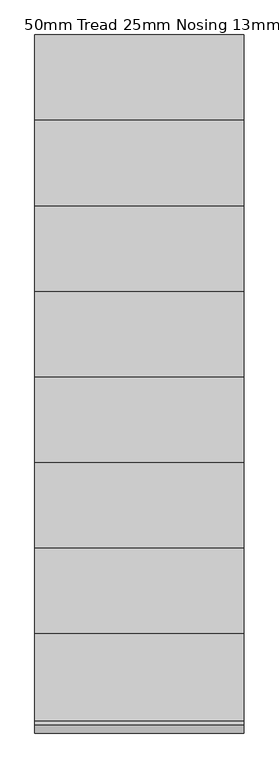
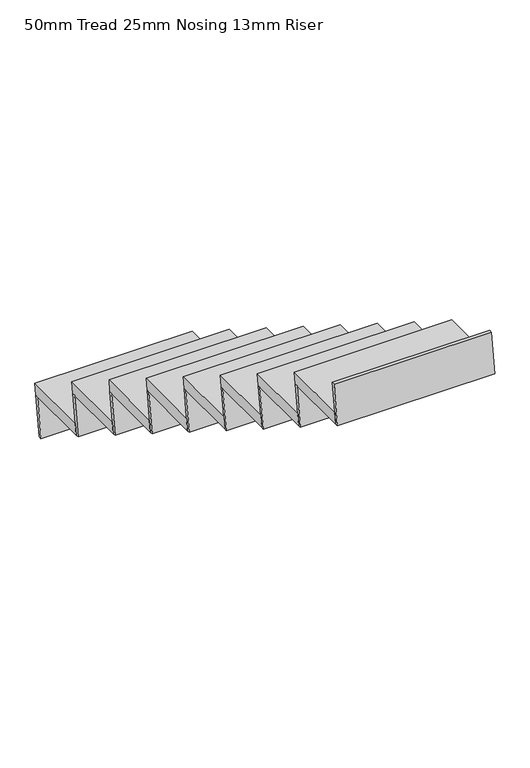
"""IFC4 building model written with IfcOpenShell, lengths in millimetres: stair flight geometry, 50mm Tread 25mm Nosing 13mm Riser."""

from ifc_helpers import new_model, si_unit, frame, origin, place, context, project, spatial, polyline, outline, extrude, source, transform, mapped, element, save


def stair_flight_50mm_tread_25mm_nosing_13mm_riser_fd2cf019(model_context):
    return source(origin(), model_context, "Body", "SweptSolid", [
        extrude(outline(polyline([(7051.2805518, 1913.0434783), (7351.2805518, 1913.0434783), (7344.0930518, 1863.0434783), (7044.0930518, 1863.0434783), (7051.2805518, 1913.0434783)])), frame((602.1868738, 0.0, 0.0), z_axis=(1.0, 0.0, 0.0), x_axis=(0.0, 1.0, 0.0)), (0.0, 0.0, 1.0), 673.3917263),
        extrude(outline(polyline([(7344.0930518, 1863.0434783), (7319.0930518, 1689.1304348), (7306.4645618, 1689.1304348), (7331.4645618, 1863.0434783), (7344.0930518, 1863.0434783)])), frame((602.1868738, 0.0, 0.0), z_axis=(1.0, 0.0, 0.0), x_axis=(0.0, 1.0, 0.0)), (0.0, 0.0, 1.0), 673.3917263),
        extrude(outline(polyline([(7069.0930518, 2036.9565217), (7044.0930518, 1863.0434783), (7031.4645618, 1863.0434783), (7056.4645618, 2036.9565217), (7069.0930518, 2036.9565217)])), frame((602.1868738, 0.0, 0.0), z_axis=(1.0, 0.0, 0.0), x_axis=(0.0, 1.0, 0.0)), (0.0, 0.0, 1.0), 673.3917263),
        extrude(outline(polyline([(6776.2805518, 2086.9565217), (7076.2805518, 2086.9565217), (7069.0930518, 2036.9565217), (6769.0930518, 2036.9565217), (6776.2805518, 2086.9565217)])), frame((602.1868738, 0.0, 0.0), z_axis=(1.0, 0.0, 0.0), x_axis=(0.0, 1.0, 0.0)), (0.0, 0.0, 1.0), 673.3917263),
        extrude(outline(polyline([(6794.0930518, 2210.8695652), (6769.0930518, 2036.9565217), (6756.4645618, 2036.9565217), (6781.4645618, 2210.8695652), (6794.0930518, 2210.8695652)])), frame((602.1868738, 0.0, 0.0), z_axis=(1.0, 0.0, 0.0), x_axis=(0.0, 1.0, 0.0)), (0.0, 0.0, 1.0), 673.3917263),
        extrude(outline(polyline([(6501.2805518, 2260.8695652), (6801.2805518, 2260.8695652), (6794.0930518, 2210.8695652), (6494.0930518, 2210.8695652), (6501.2805518, 2260.8695652)])), frame((602.1868738, 0.0, 0.0), z_axis=(1.0, 0.0, 0.0), x_axis=(0.0, 1.0, 0.0)), (0.0, 0.0, 1.0), 673.3917263),
        extrude(outline(polyline([(6519.0930518, 2384.7826087), (6494.0930518, 2210.8695652), (6481.4645618, 2210.8695652), (6506.4645618, 2384.7826087), (6519.0930518, 2384.7826087)])), frame((602.1868738, 0.0, 0.0), z_axis=(1.0, 0.0, 0.0), x_axis=(0.0, 1.0, 0.0)), (0.0, 0.0, 1.0), 673.3917263),
        extrude(outline(polyline([(6226.2805518, 2434.7826087), (6526.2805518, 2434.7826087), (6519.0930518, 2384.7826087), (6219.0930518, 2384.7826087), (6226.2805518, 2434.7826087)])), frame((602.1868738, 0.0, 0.0), z_axis=(1.0, 0.0, 0.0), x_axis=(0.0, 1.0, 0.0)), (0.0, 0.0, 1.0), 673.3917263),
        extrude(outline(polyline([(6244.0930518, 2558.6956522), (6219.0930518, 2384.7826087), (6206.4645618, 2384.7826087), (6231.4645618, 2558.6956522), (6244.0930518, 2558.6956522)])), frame((602.1868738, 0.0, 0.0), z_axis=(1.0, 0.0, 0.0), x_axis=(0.0, 1.0, 0.0)), (0.0, 0.0, 1.0), 673.3917263),
        extrude(outline(polyline([(5951.2805518, 2608.6956522), (6251.2805518, 2608.6956522), (6244.0930518, 2558.6956522), (5944.0930518, 2558.6956522), (5951.2805518, 2608.6956522)])), frame((602.1868738, 0.0, 0.0), z_axis=(1.0, 0.0, 0.0), x_axis=(0.0, 1.0, 0.0)), (0.0, 0.0, 1.0), 673.3917263),
        extrude(outline(polyline([(5969.0930518, 2732.6086957), (5944.0930518, 2558.6956522), (5931.4645618, 2558.6956522), (5956.4645618, 2732.6086957), (5969.0930518, 2732.6086957)])), frame((602.1868738, 0.0, 0.0), z_axis=(1.0, 0.0, 0.0), x_axis=(0.0, 1.0, 0.0)), (0.0, 0.0, 1.0), 673.3917263),
        extrude(outline(polyline([(5676.2805518, 2782.6086957), (5976.2805518, 2782.6086957), (5969.0930518, 2732.6086957), (5669.0930518, 2732.6086957), (5676.2805518, 2782.6086957)])), frame((602.1868738, 0.0, 0.0), z_axis=(1.0, 0.0, 0.0), x_axis=(0.0, 1.0, 0.0)), (0.0, 0.0, 1.0), 673.3917263),
        extrude(outline(polyline([(5694.0930518, 2906.5217391), (5669.0930518, 2732.6086957), (5656.4645618, 2732.6086957), (5681.4645618, 2906.5217391), (5694.0930518, 2906.5217391)])), frame((602.1868738, 0.0, 0.0), z_axis=(1.0, 0.0, 0.0), x_axis=(0.0, 1.0, 0.0)), (0.0, 0.0, 1.0), 673.3917263),
        extrude(outline(polyline([(5401.2805518, 2956.5217391), (5701.2805518, 2956.5217391), (5694.0930518, 2906.5217391), (5394.0930518, 2906.5217391), (5401.2805518, 2956.5217391)])), frame((602.1868738, 0.0, 0.0), z_axis=(1.0, 0.0, 0.0), x_axis=(0.0, 1.0, 0.0)), (0.0, 0.0, 1.0), 673.3917263),
        extrude(outline(polyline([(5419.0930518, 3080.4347826), (5394.0930518, 2906.5217391), (5381.4645618, 2906.5217391), (5406.4645618, 3080.4347826), (5419.0930518, 3080.4347826)])), frame((602.1868738, 0.0, 0.0), z_axis=(1.0, 0.0, 0.0), x_axis=(0.0, 1.0, 0.0)), (0.0, 0.0, 1.0), 673.3917263),
        extrude(outline(polyline([(5144.0930518, 3254.3478261), (5119.0930518, 3080.4347826), (5106.4645618, 3080.4347826), (5131.4645618, 3254.3478261), (5144.0930518, 3254.3478261)])), frame((602.1868738, 0.0, 0.0), z_axis=(1.0, 0.0, 0.0), x_axis=(0.0, 1.0, 0.0)), (0.0, 0.0, 1.0), 673.3917263),
        extrude(outline(polyline([(5126.2805518, 3130.4347826), (5426.2805518, 3130.4347826), (5419.0930518, 3080.4347826), (5119.0930518, 3080.4347826), (5126.2805518, 3130.4347826)])), frame((602.1868738, 0.0, 0.0), z_axis=(1.0, 0.0, 0.0), x_axis=(0.0, 1.0, 0.0)), (0.0, 0.0, 1.0), 673.3917263),
    ])


if __name__ == "__main__":
    model = new_model("IFC4")
    model_context = context("Model", 3, world=origin())
    ifc_project = project(units=[si_unit("LENGTHUNIT", "METRE", prefix="MILLI")], contexts=[model_context])
    site = spatial("IfcSite", under=ifc_project)
    building = spatial("IfcBuilding", under=site)
    placement = place(None, origin())
    stair_flight_50mm_tread_25mm_nosing_13mm_riser_shape = stair_flight_50mm_tread_25mm_nosing_13mm_riser_fd2cf019(model_context)
    element("IfcStairFlight", 1, ObjectType="50mm Tread 25mm Nosing 13mm Riser", at=placement, inside=building, context=model_context, shape_type="MappedRepresentation", body=[
        mapped(stair_flight_50mm_tread_25mm_nosing_13mm_riser_shape, transform((0.0, 0.0, 0.0), x_axis=(1.0, 0.0, 0.0), y_axis=(0.0, 1.0, 0.0), z_axis=(0.0, 0.0, 1.0))),
    ])
    save(model, "model.ifc")
